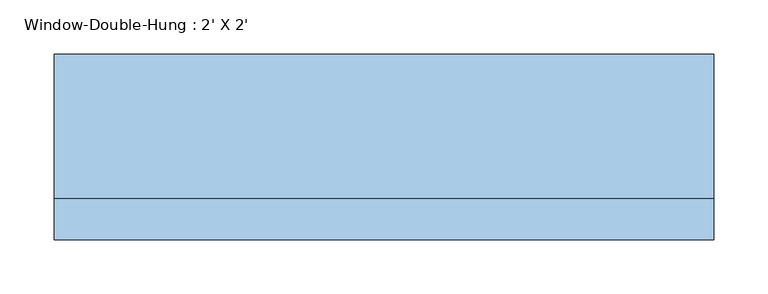
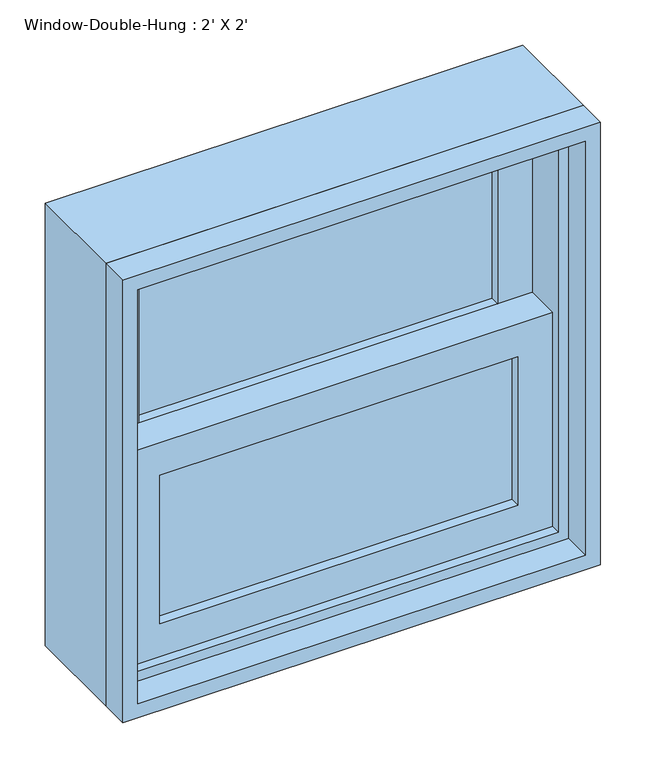
"""IFC4 building model written with IfcOpenShell, lengths in millimetres: window geometry, Window-Double-Hung : 2' X 2'."""

from ifc_helpers import new_model, si_unit, frame, origin, place, context, project, spatial, polyline, outline, extrude, source, transform, mapped, element, save


def window_double_hung_2_x_2_0206a36d(model_context):
    return source(origin(), model_context, "Body", "SweptSolid", [
        extrude(outline(polyline([(228.6, 6.35), (228.6, 0.0), (-228.6, 0.0), (-228.6, 6.35), (228.6, 6.35)])), frame((0.0, 0.0, 990.6), z_axis=(0.0, 0.0, 1.0), x_axis=(1.0, 0.0, 0.0)), (0.0, 0.0, 1.0), 200.025),
        extrude(outline(polyline([(-228.6, -6.35), (228.6, -6.35), (228.6, -12.7), (-228.6, -12.7), (-228.6, -6.35)])), frame((0.0, 0.0, 990.6), z_axis=(0.0, 0.0, 1.0), x_axis=(1.0, 0.0, 0.0)), (0.0, 0.0, 1.0), 200.025),
        extrude(outline(polyline([(228.6, 50.8), (228.6, 44.45), (-228.6, 44.45), (-228.6, 50.8), (228.6, 50.8)])), frame((0.0, 0.0, 1235.075), z_axis=(0.0, 0.0, 1.0), x_axis=(1.0, 0.0, 0.0)), (0.0, 0.0, 1.0), 200.025),
        extrude(outline(polyline([(-228.6, 38.1), (228.6, 38.1), (228.6, 31.75), (-228.6, 31.75), (-228.6, 38.1)])), frame((0.0, 0.0, 1235.075), z_axis=(0.0, 0.0, 1.0), x_axis=(1.0, 0.0, 0.0)), (0.0, 0.0, 1.0), 200.025),
        extrude(outline(polyline([(1235.075, -273.05), (946.15, -273.05), (946.15, 273.05), (1235.075, 273.05), (1235.075, -273.05)]), holes=[polyline([(1190.625, 228.6), (990.6, 228.6), (990.6, -228.6), (1190.625, -228.6), (1190.625, 228.6)])]), frame((0.0, -25.4, 0.0), z_axis=(0.0, 1.0, 0.0), x_axis=(0.0, 0.0, 1.0)), (0.0, 0.0, 1.0), 44.45),
        extrude(outline(polyline([(1479.55, -273.05), (1190.625, -273.05), (1190.625, 273.05), (1479.55, 273.05), (1479.55, -273.05)]), holes=[polyline([(1435.1, 228.6), (1235.075, 228.6), (1235.075, -228.6), (1435.1, -228.6), (1435.1, 228.6)])]), frame((0.0, 19.05, 0.0), z_axis=(0.0, 1.0, 0.0), x_axis=(0.0, 0.0, 1.0)), (0.0, 0.0, 1.0), 44.45),
        extrude(outline(polyline([(1511.3, -304.8), (914.4, -304.8), (914.4, 304.8), (1511.3, 304.8), (1511.3, -304.8)]), holes=[polyline([(1479.55, 273.05), (946.15, 273.05), (946.15, -273.05), (1479.55, -273.05), (1479.55, 273.05)])]), frame((0.0, -38.1, 0.0), z_axis=(0.0, 1.0, 0.0), x_axis=(0.0, 0.0, 1.0)), (0.0, 0.0, 1.0), 133.35),
        extrude(outline(polyline([(1511.3, 304.8), (1511.3, -304.8), (914.4, -304.8), (914.4, 304.8), (1511.3, 304.8)]), holes=[polyline([(1492.25, 285.75), (933.45, 285.75), (933.45, -285.75), (1492.25, -285.75), (1492.25, 285.75)])]), frame((0.0, -76.2, 0.0), z_axis=(0.0, 1.0, 0.0), x_axis=(0.0, 0.0, 1.0)), (0.0, 0.0, 1.0), 38.1),
    ])


if __name__ == "__main__":
    model = new_model("IFC4")
    model_context = context("Model", 3, world=origin())
    ifc_project = project(units=[si_unit("LENGTHUNIT", "METRE", prefix="MILLI")], contexts=[model_context])
    site = spatial("IfcSite", under=ifc_project)
    building = spatial("IfcBuilding", under=site)
    placement = place(None, origin())
    window_double_hung_2_x_2_shape = window_double_hung_2_x_2_0206a36d(model_context)
    element("IfcWindow", 1, ObjectType="Window-Double-Hung : 2' X 2'", at=placement, inside=building, context=model_context, shape_type="MappedRepresentation", body=[
        mapped(window_double_hung_2_x_2_shape, transform((0.0, 0.0, 0.0), x_axis=(1.0, 0.0, 0.0), y_axis=(0.0, 1.0, 0.0), z_axis=(0.0, 0.0, 1.0))),
    ])
    save(model, "model.ifc")

# Revit data of these elements
# Type "Window-Double-Hung : 2' X 2'"
#   Type Mark = "25"
#   Fire Rating = "0.5h"
#   Construction Type Id = "DG-DR"
#   Assembly Code = "B2020100"
#   Analytic Construction = "Double glazing - domestic"
#   Wall Thickness [instance default] = 0' - 6"
#   Window Inset [instance default] = 0' - 0"
#   Visual Light Transmittance = 0.81
#   Thermal Resistance (R) = 1.8146 (h·ft²·°F)/BTU
#   Solar Heat Gain Coefficient = 0.76
#   Muntin Width = 1' - 6"
#   Muntin Height = 0' - 7 7/8"
#   Interior Wall Closure [instance default] = 0' - 1 1/2"
#   Rough Width = 2' - 0 1/2"
#   Rough Height = 2' - 0"
#   Frame Extension [instance default] = 0' - 1 1/4"
#   Exterior Wall Closure [instance default] = 0' - 0 1/2"
#   Extension Jamb [instance default] = 0' - 1 1/2"
#   Heat Transfer Coefficient (U) = 0.5511 BTU/(h·ft²·°F)
#   Height = 1' - 11 1/2"
#   Width = 2' - 0"
#   Top Muntin Visibility = yes
#   Indicator Visibility [instance default] = yes
#   Extension Jamb Visibility [instance default] = yes
#   Interior Trim Visibility [instance default] = yes
#   Exterior Trim Visibility [instance default] = yes
#   Define Thermal Properties by = 1
#   Bottom Muntin Visibility = yes
#   Muntin Pattern = Muntin Pattern_2x2 : Muntin Pattern_2x2
#   Interior Trim Material = Wood - Stained
#   Interior Trim = Trim-Window-Interior-Flat : Picture Frame
#   Exterior Trim Material = Clad - White
#   Exterior Trim = Trim-Window-Exterior-Flat : with Sill
#   Glass Panel Material = Glass
#   Exterior Frame Material = Clad - White
#   Interior Frame Material = Wood - Stained
#   Wall Closure = (empty or 0)
# Element 1 (IfcWindow, "Window-Double-Hung : 2' X 2'")
#   Materials on its faces: "Wood - Stained", "Glass", "Clad - White"
# Materials
#   "Wood - Stained": class "Wood", colour RGB 224 178 126, transparency 0, Cost = 0
#   "Clad - White": class "Wood", colour RGB 242 242 238, transparency 0, Cost = 0
#   "Glass": class "Glass", colour RGB 0 128 192, transparency 0.75, Description = "Soda Lime Glass", Cost = 0
